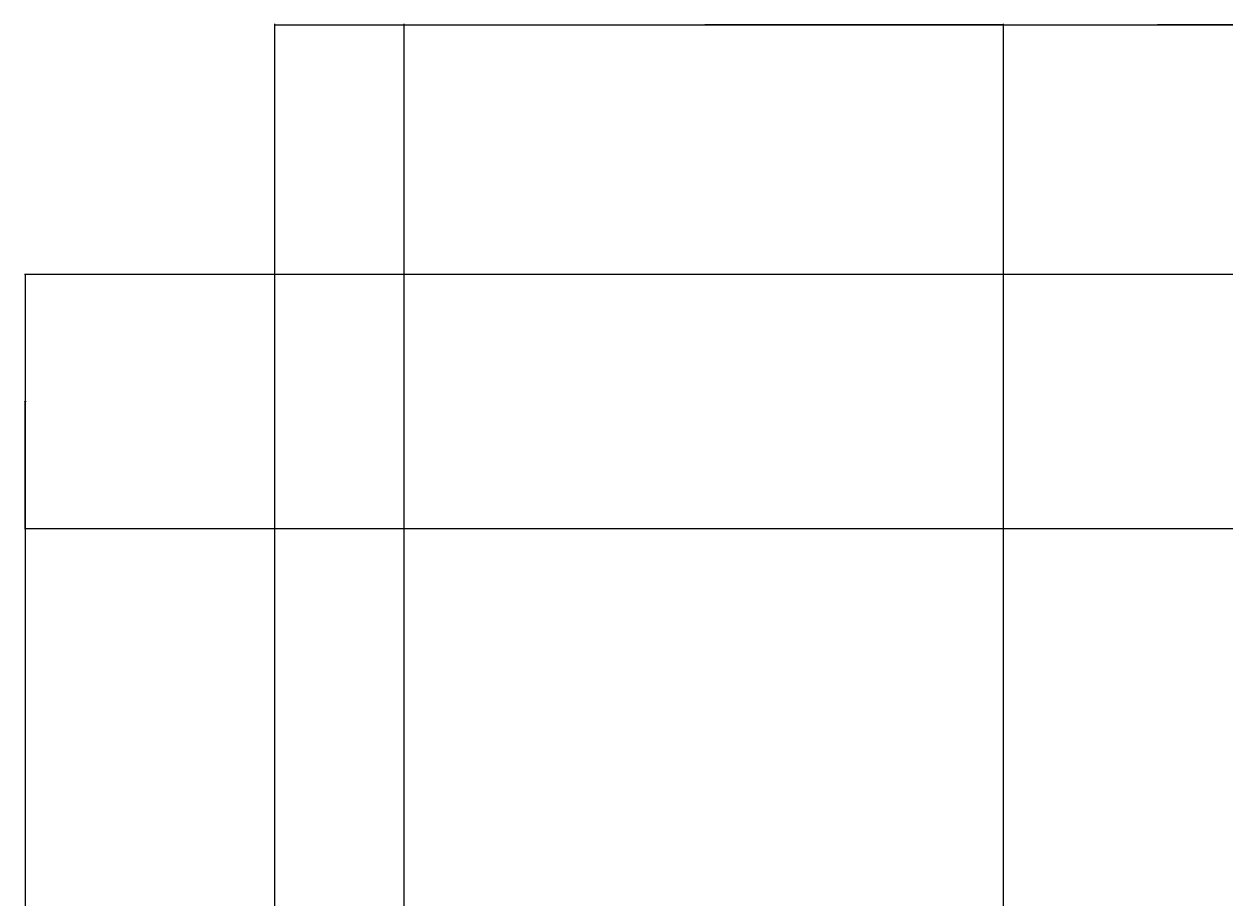
# Model space of a CAD drawing. Units: inches. Extents: x 1693 to 2974, y 2201 to 2965.
# Tile 7 of 24: x 1693 to 1976, y 2759 to 2965. Entities that reach past the tile are written whole.
import ezdxf

# ---------------------------------------------------------------- set-up
doc = ezdxf.new("R2010")
doc.units = ezdxf.units.IN
doc.header["$LTSCALE"] = 2
doc.header["$MEASUREMENT"] = 0
doc.layers.add('A-ANNO-DIMS', color=2, linetype='Continuous', lineweight=18)
doc.styles.get("Standard").update_dxf_attribs({"font": 'arial.ttf'})
doc.dimstyles.get("Standard").update_dxf_attribs({"dimtxt": 0.18, "dimasz": 0.18, "dimexe": 0.18, "dimexo": 0.0625, "dimgap": 0.09, "dimtad": 0, "dimtih": 1, "dimtoh": 1, "dimdec": 1, "dimzin": 0, "dimdsep": 46, "dimlunit": 3, "dimtxsty": 'Standard', "dimcen": 0.09, "dimadec": 0, "dimazin": 0, "dimtfac": 1, "dimtdec": 1, "dimtofl": 0, "dimtmove": 0, "dimatfit": 3, "dimfxl": 1, "dimtolj": 1, "dimtzin": 0, "dimarcsym": 0})

# ---------------------------------------------------------------- blocks, each defined once
blk = doc.blocks.new('*D81')
at = {"layer": 'A-ANNO-DIMS', "color": 0, "lineweight": -2, "ltscale": 2, "transparency": 16777216}
for p, q in [((1752.34, 2553.91), (1752.34, 2964.96)), ((1752.52, 2964.78), (2332.94, 2964.78)), ((2914.06, 2964.78), (2333.64, 2964.78)), ((2914.24, 2754.97), (2914.24, 2964.96))]:
    blk.add_line(p, q, dxfattribs=at)
at = {"layer": 'A-ANNO-DIMS', "color": 0, "ltscale": 2, "transparency": 16777216}
for points in [[(1752.52, 2964.81), (1752.52, 2964.75), (1752.34, 2964.78)], [(2914.06, 2964.81), (2914.06, 2964.75), (2914.24, 2964.78)]]:
    blk.add_solid(points, dxfattribs=at)
at = {"layer": 'Defpoints', "color": 0, "ltscale": 2, "transparency": 16777216}
for p in [(2914.24, 2964.78), (2914.24, 2754.9), (1752.34, 2553.84)]:
    blk.add_point(p, dxfattribs=at)
at = {"layer": 'A-ANNO-DIMS', "color": 0, "ltscale": 2, "transparency": 16777216, "insert": (2333.29, 2964.78), "char_height": 0.18, "attachment_point": 5}
blk.add_mtext('\\A1;1162', dxfattribs=at)
blk = doc.blocks.new('*D82')
at = {"layer": 'A-ANNO-DIMS', "color": 0, "lineweight": -2, "ltscale": 2, "transparency": 16777216}
for p, q in [((2615.67, 2906.08), (1693.46, 2906.08)), ((1693.64, 2905.9), (1693.64, 2582.94)), ((1693.64, 2259.62), (1693.64, 2582.58)), ((2096.17, 2259.44), (1693.46, 2259.44))]:
    blk.add_line(p, q, dxfattribs=at)
at = {"layer": 'A-ANNO-DIMS', "color": 0, "ltscale": 2, "transparency": 16777216}
for points in [[(1693.61, 2905.9), (1693.67, 2905.9), (1693.64, 2906.08)], [(1693.61, 2259.62), (1693.67, 2259.62), (1693.64, 2259.44)]]:
    blk.add_solid(points, dxfattribs=at)
at = {"layer": 'Defpoints', "color": 0, "ltscale": 2, "transparency": 16777216}
for p in [(1693.64, 2906.08), (2615.74, 2906.08), (2096.24, 2259.44)]:
    blk.add_point(p, dxfattribs=at)
at = {"layer": 'A-ANNO-DIMS', "color": 0, "ltscale": 2, "transparency": 16777216, "insert": (1693.64, 2582.76), "char_height": 0.18, "attachment_point": 5}
blk.add_mtext('\\A1;646.6', dxfattribs=at)
blk = doc.blocks.new('*D91')
at = {"layer": 'A-ANNO-DIMS', "color": 0, "lineweight": -2, "ltscale": 2, "transparency": 16777216}
for p, q in [((2615.67, 2906.08), (1693.46, 2906.08)), ((1693.64, 2905.9), (1693.64, 2876.35)), ((1693.64, 2846.43), (1693.64, 2875.98)), ((2479.17, 2846.25), (1693.46, 2846.25))]:
    blk.add_line(p, q, dxfattribs=at)
at = {"layer": 'A-ANNO-DIMS', "color": 0, "ltscale": 2, "transparency": 16777216}
for points in [[(1693.61, 2905.9), (1693.67, 2905.9), (1693.64, 2906.08)], [(1693.61, 2846.43), (1693.67, 2846.43), (1693.64, 2846.25)]]:
    blk.add_solid(points, dxfattribs=at)
at = {"layer": 'Defpoints', "color": 0, "ltscale": 2, "transparency": 16777216}
for p in [(2615.74, 2906.08), (1693.64, 2846.25), (2479.24, 2846.25)]:
    blk.add_point(p, dxfattribs=at)
at = {"layer": 'A-ANNO-DIMS', "color": 0, "ltscale": 2, "transparency": 16777216, "insert": (1693.64, 2876.17), "char_height": 0.18, "attachment_point": 5}
blk.add_mtext('\\A1;59.82', dxfattribs=at)
blk = doc.blocks.new('*D102')
at = {"layer": 'A-ANNO-DIMS', "color": 0, "lineweight": -2, "ltscale": 2, "transparency": 16777216}
for p, q in [((1782.74, 2706.91), (1782.74, 2964.96)), ((1782.92, 2964.78), (1852.97, 2964.78)), ((1923.56, 2964.78), (1853.5, 2964.78)), ((1923.74, 2706.91), (1923.74, 2964.96))]:
    blk.add_line(p, q, dxfattribs=at)
at = {"layer": 'A-ANNO-DIMS', "color": 0, "ltscale": 2, "transparency": 16777216}
for points in [[(1782.92, 2964.81), (1782.92, 2964.75), (1782.74, 2964.78)], [(1923.56, 2964.81), (1923.56, 2964.75), (1923.74, 2964.78)]]:
    blk.add_solid(points, dxfattribs=at)
at = {"layer": 'Defpoints', "color": 0, "ltscale": 2, "transparency": 16777216}
for p in [(1923.74, 2964.78), (1782.74, 2706.84), (1923.74, 2706.84)]:
    blk.add_point(p, dxfattribs=at)
at = {"layer": 'A-ANNO-DIMS', "color": 0, "ltscale": 2, "transparency": 16777216, "insert": (1853.24, 2964.78), "char_height": 0.18, "attachment_point": 5}
blk.add_mtext('\\A1;141', dxfattribs=at)
blk = doc.blocks.new('*D103')
at = {"layer": 'A-ANNO-DIMS', "color": 0, "lineweight": -2, "ltscale": 2, "transparency": 16777216}
for p, q in [((1923.74, 2737.28), (1923.74, 2964.96)), ((1923.92, 2964.78), (1959.52, 2964.78)), ((1995.56, 2964.78), (1959.95, 2964.78)), ((1995.74, 2737.28), (1995.74, 2964.96))]:
    blk.add_line(p, q, dxfattribs=at)
at = {"layer": 'A-ANNO-DIMS', "color": 0, "ltscale": 2, "transparency": 16777216}
for points in [[(1923.92, 2964.81), (1923.92, 2964.75), (1923.74, 2964.78)], [(1995.56, 2964.81), (1995.56, 2964.75), (1995.74, 2964.78)]]:
    blk.add_solid(points, dxfattribs=at)
at = {"layer": 'Defpoints', "color": 0, "ltscale": 2, "transparency": 16777216}
for p in [(1995.74, 2964.78), (1923.74, 2737.22), (1995.74, 2737.22)]:
    blk.add_point(p, dxfattribs=at)
at = {"layer": 'A-ANNO-DIMS', "color": 0, "ltscale": 2, "transparency": 16777216, "insert": (1959.74, 2964.78), "char_height": 0.18, "attachment_point": 5}
blk.add_mtext('\\A1;72', dxfattribs=at)

msp = doc.modelspace()

# ---------------------------------------------------------------- dimensions: what is measured, and where the dimension line sits
at = {"layer": 'A-ANNO-DIMS', "ltscale": 2}
for base, p1, p2, picture, middle in [((2914.2363, 2964.7761), (1752.3363, 2553.8449), (2914.2363, 2754.903), '*D81', (2333.2863, 2964.7761)), ((1923.7363, 2964.7761), (1782.7363, 2706.8449), (1923.7363, 2706.8449), '*D102', (1853.2363, 2964.7761)), ((1995.7363, 2964.7761), (1923.7363, 2737.2161), (1995.7363, 2737.2161), '*D103', (1959.7363, 2964.7761))]:
    dim = msp.add_linear_dim(base=base, p1=p1, p2=p2, dimstyle='Standard', override={"dimdec": 0, "dimlfac": 1, "dimrnd": 0, "dimzin": 0, "dimdsep": 46, "dimlunit": 2}, dxfattribs=at)
    dim.commit()
    dim.dimension.update_dxf_attribs({"geometry": picture, "text_midpoint": middle})
for base, p1, p2, override, picture, middle in [((1693.6363, 2906.0761), (2096.2363, 2259.4449), (2615.7363, 2906.0761), {"dimdec": 1, "dimlfac": 1, "dimrnd": 0, "dimzin": 0, "dimdsep": 46, "dimlunit": 2}, '*D82', (1693.6363, 2582.7605)), ((1693.6363, 2846.2547), (2615.7363, 2906.0761), (2479.2363, 2846.2547), {"dimdec": 2, "dimlfac": 1, "dimrnd": 0, "dimzin": 0, "dimdsep": 46, "dimlunit": 2}, '*D91', (1693.6363, 2876.1654))]:
    dim = msp.add_linear_dim(base=base, p1=p1, p2=p2, angle=90, dimstyle='Standard', override=override, dxfattribs=at)
    dim.commit()
    dim.dimension.update_dxf_attribs({"geometry": picture, "text_midpoint": middle})

doc.saveas('drawing.dxf')
